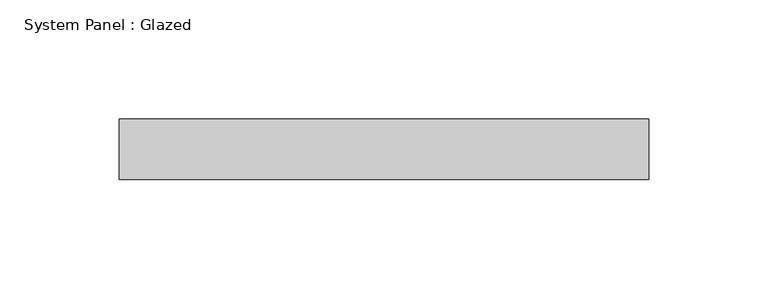
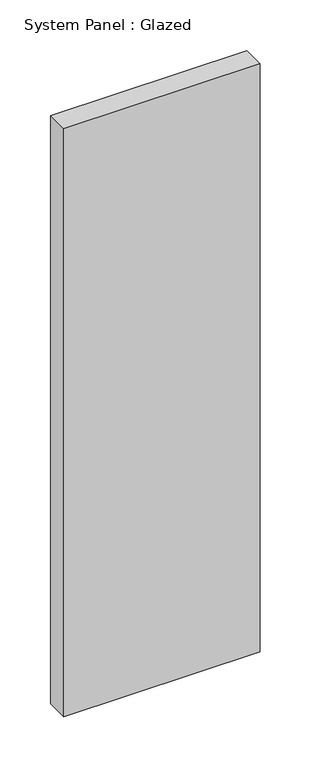
"""IFC4 building model written with IfcOpenShell, lengths in millimetres: plate geometry, System Panel : Glazed."""

from ifc_helpers import new_model, si_unit, origin, origin_with_axes, place, context, project, spatial, polyline, outline, extrude, source, transform, mapped, element, save


def system_panel_glazed_0590c333(model_context):
    return source(origin(), model_context, "Body", "SweptSolid", [
        extrude(outline(polyline([(111.125, 19.05), (-111.125, 19.05), (-111.125, 44.45), (111.125, 44.45), (111.125, 19.05)])), origin_with_axes(), (0.0, 0.0, 1.0), 704.5046847),
    ])


if __name__ == "__main__":
    model = new_model("IFC4")
    model_context = context("Model", 3, world=origin())
    ifc_project = project(units=[si_unit("LENGTHUNIT", "METRE", prefix="MILLI")], contexts=[model_context])
    site = spatial("IfcSite", under=ifc_project)
    building = spatial("IfcBuilding", under=site)
    placement = place(None, origin())
    system_panel_glazed_shape = system_panel_glazed_0590c333(model_context)
    element("IfcPlate", 1, ObjectType="System Panel : Glazed", at=placement, inside=building, context=model_context, shape_type="MappedRepresentation", body=[
        mapped(system_panel_glazed_shape, transform((0.0, 0.0, 0.0), x_axis=(1.0, 0.0, 0.0), y_axis=(0.0, 1.0, 0.0), z_axis=(0.0, 0.0, 1.0))),
    ])
    save(model, "model.ifc")

# Revit data of these elements
# Type "System Panel : Glazed"
#   Construction Type Id = "GSP4R"
#   Analytic Construction = "1/8 in Pilkington single glazing"
#   Visual Light Transmittance = 0.9
#   Solar Heat Gain Coefficient = 0.86
#   Heat Transfer Coefficient (U) = 1.18115 BTU/(h·ft²·°F)
#   Define Thermal Properties by = 1
# Element 1 (IfcPlate, "System Panel : Glazed")
#   Materials on its faces: "Glass"
# Materials
#   "Glass": class "Glass", colour RGB 0 128 192, transparency 0.75, Description = "Soda Lime Glass", Cost = 0
